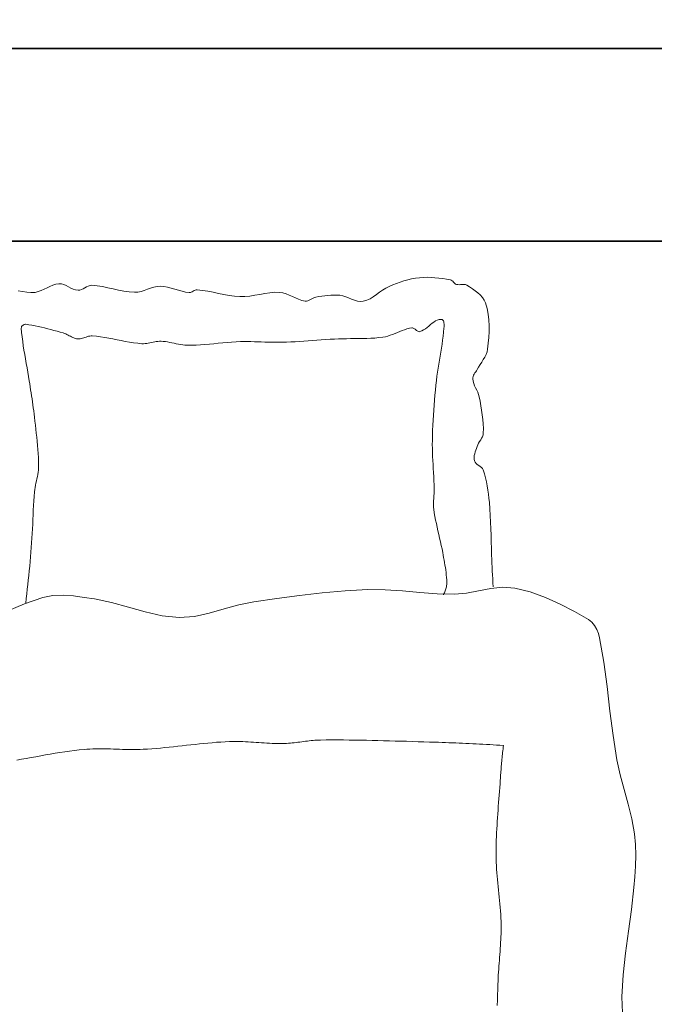
# Model space of a CAD drawing. Units: inches. Extents: x -36302355 to 648, y -221479757 to 75.
# Tile 35 of 37: x 311 to 341, y -20 to 26. Entities that reach past the tile are written whole.
import ezdxf

# ---------------------------------------------------------------- set-up
doc = ezdxf.new("R2010")
doc.units = ezdxf.units.IN
doc.header["$MEASUREMENT"] = 0
for name, color, linetype, lineweight in [('A-ANNO-DIMS', 2, 'Continuous', 18), ('A-FURN', 8, 'Continuous', 13), ('A-WALL', 7, 'Continuous', 35)]:
    doc.layers.add(name, color=color, linetype=linetype, lineweight=lineweight)
doc.styles.get("Standard").update_dxf_attribs({"font": 'arial.ttf'})
doc.dimstyles.get("Standard").update_dxf_attribs({"dimtxt": 0.18, "dimasz": 0.18, "dimexe": 0.18, "dimexo": 0.0625, "dimgap": 0.09, "dimtad": 0, "dimtih": 1, "dimtoh": 1, "dimdec": 0, "dimzin": 0, "dimdsep": 46, "dimlunit": 3, "dimtxsty": 'Standard', "dimcen": 0.09, "dimadec": 0, "dimazin": 0, "dimtfac": 1, "dimtdec": 0, "dimtofl": 0, "dimtmove": 0, "dimatfit": 3, "dimfxl": 1, "dimtolj": 1, "dimtzin": 0, "dimarcsym": 0})

# ---------------------------------------------------------------- blocks, each defined once
blk = doc.blocks.new('*D4')
at = {"layer": 'A-ANNO-DIMS', "color": 0, "lineweight": -2, "transparency": 16777216}
for p, q in [((145.197, 25.043), (145.197, 71.11)), ((145.377, 70.93), (364.803, 70.93)), ((605.017, 70.93), (385.59, 70.93)), ((605.197, 25.043), (605.197, 71.11))]:
    blk.add_line(p, q, dxfattribs=at)
at = {"layer": 'A-ANNO-DIMS', "color": 0, "transparency": 16777216}
for points in [[(145.377, 70.96), (145.377, 70.9), (145.197, 70.93)], [(605.017, 70.96), (605.017, 70.9), (605.197, 70.93)]]:
    blk.add_solid(points, dxfattribs=at)
at = {"layer": 'Defpoints', "color": 0, "transparency": 16777216}
for p in [(605.197, 70.93), (145.197, 24.981), (605.197, 24.981)]:
    blk.add_point(p, dxfattribs=at)
at = {"layer": 'A-ANNO-DIMS', "color": 0, "transparency": 16777216, "insert": (375.197, 70.93), "char_height": 6, "attachment_point": 5}
blk.add_mtext('\\A1;38\'-4"', dxfattribs=at)
blk = doc.blocks.new('BED-DOUBLE')
for p, q in [((29.019, 79.595), (28.885, 79.529)), ((29.156, 79.653), (29.019, 79.595)), ((29.295, 79.695), (29.156, 79.653)), ((29.439, 79.716), (29.295, 79.695)), ((29.555, 79.707), (29.439, 79.716)), ((29.667, 79.676), (29.555, 79.707)), ((29.776, 79.63), (29.667, 79.676)), ((29.885, 79.575), (29.776, 79.63)), ((30.811, 79.61), (30.732, 79.571)), ((30.892, 79.636), (30.811, 79.61)), ((30.976, 79.644), (30.892, 79.636)), ((31.228, 79.624), (30.976, 79.644)), ((31.477, 79.585), (31.228, 79.624)), ((34.02, 79.587), (33.869, 79.555)), ((34.173, 79.598), (34.02, 79.587)), ((34.345, 79.587), (34.173, 79.598)), ((34.515, 79.557), (34.345, 79.587)), ((44.859, 79.595), (44.703, 79.516)), ((45.03, 79.665), (44.859, 79.595)), ((45.203, 79.731), (45.03, 79.665)), ((45.378, 79.793), (45.203, 79.731)), ((45.554, 79.85), (45.378, 79.793)), ((45.733, 79.9), (45.554, 79.85)), ((45.912, 79.943), (45.733, 79.9)), ((46.094, 79.977), (45.912, 79.943)), ((46.276, 80.001), (46.094, 79.977)), ((46.457, 80.015), (46.276, 80.001)), ((46.638, 80.019), (46.457, 80.015)), ((46.819, 80.013), (46.638, 80.019)), ((47.001, 80.001), (46.819, 80.013)), ((47.182, 79.981), (47.001, 80.001)), ((47.363, 79.957), (47.182, 79.981)), ((47.542, 79.928), (47.363, 79.957)), ((47.721, 79.897), (47.542, 79.928)), ((47.762, 79.883), (47.721, 79.897)), ((47.799, 79.86), (47.762, 79.883)), ((47.832, 79.831), (47.799, 79.86)), ((47.865, 79.797), (47.832, 79.831)), ((47.897, 79.763), (47.865, 79.797)), ((47.93, 79.732), (47.897, 79.763)), ((47.966, 79.705), (47.93, 79.732)), ((48.005, 79.687), (47.966, 79.705)), ((48.065, 79.675), (48.005, 79.687)), ((48.126, 79.673), (48.065, 79.675)), ((48.189, 79.677), (48.126, 79.673)), ((48.253, 79.684), (48.189, 79.677)), ((48.316, 79.688), (48.253, 79.684)), ((48.376, 79.687), (48.316, 79.688)), ((48.434, 79.676), (48.376, 79.687)), ((48.487, 79.652), (48.434, 79.676)), ((48.617, 79.57), (48.487, 79.652)), ((27.733, 79.348), (27.532, 79.381)), ((27.935, 79.319), (27.733, 79.348)), ((28.135, 79.305), (27.935, 79.319)), ((28.332, 79.316), (28.135, 79.305)), ((28.475, 79.348), (28.332, 79.316)), ((28.614, 79.399), (28.475, 79.348)), ((28.75, 79.461), (28.614, 79.399)), ((28.885, 79.529), (28.75, 79.461)), ((29.994, 79.518), (29.885, 79.575)), ((30.103, 79.467), (29.994, 79.518)), ((30.215, 79.429), (30.103, 79.467)), ((30.331, 79.412), (30.215, 79.429)), ((30.415, 79.419), (30.331, 79.412)), ((30.496, 79.445), (30.415, 79.419)), ((30.575, 79.483), (30.496, 79.445)), ((30.654, 79.527), (30.575, 79.483)), ((30.732, 79.571), (30.654, 79.527)), ((31.725, 79.534), (31.477, 79.585)), ((31.973, 79.478), (31.725, 79.534)), ((32.221, 79.421), (31.973, 79.478)), ((32.469, 79.372), (32.221, 79.421)), ((32.718, 79.336), (32.469, 79.372)), ((32.97, 79.321), (32.718, 79.336)), ((33.123, 79.331), (32.97, 79.321)), ((33.273, 79.362), (33.123, 79.331)), ((33.423, 79.406), (33.273, 79.362)), ((33.571, 79.458), (33.423, 79.406)), ((33.72, 79.51), (33.571, 79.458)), ((33.869, 79.555), (33.72, 79.51)), ((34.684, 79.516), (34.515, 79.557)), ((34.852, 79.467), (34.684, 79.516)), ((35.02, 79.416), (34.852, 79.467)), ((35.188, 79.369), (35.02, 79.416)), ((35.358, 79.33), (35.188, 79.369)), ((35.529, 79.305), (35.358, 79.33)), ((35.577, 79.308), (35.529, 79.305)), ((35.623, 79.323), (35.577, 79.308)), ((35.669, 79.345), (35.623, 79.323)), ((35.714, 79.371), (35.669, 79.345)), ((35.758, 79.398), (35.714, 79.371)), ((35.804, 79.42), (35.758, 79.398)), ((35.85, 79.435), (35.804, 79.42)), ((35.898, 79.439), (35.85, 79.435)), ((36.149, 79.41), (35.898, 79.439)), ((36.398, 79.368), (36.149, 79.41)), ((36.646, 79.318), (36.398, 79.368)), ((36.894, 79.264), (36.646, 79.318)), ((37.142, 79.212), (36.894, 79.264)), ((37.39, 79.167), (37.142, 79.212)), ((37.64, 79.133), (37.39, 79.167)), ((37.891, 79.115), (37.64, 79.133)), ((38.357, 79.144), (38.124, 79.119)), ((38.588, 79.18), (38.357, 79.144)), ((38.82, 79.223), (38.588, 79.18)), ((39.051, 79.265), (38.82, 79.223)), ((39.283, 79.299), (39.051, 79.265)), ((39.515, 79.318), (39.283, 79.299)), ((39.748, 79.315), (39.515, 79.318)), ((39.902, 79.292), (39.748, 79.315)), ((40.051, 79.248), (39.902, 79.292)), ((40.198, 79.189), (40.051, 79.248)), ((40.343, 79.122), (40.198, 79.189)), ((41.721, 79.137), (41.582, 79.116)), ((41.86, 79.157), (41.721, 79.137)), ((42, 79.173), (41.86, 79.157)), ((42.139, 79.184), (42, 79.173)), ((42.279, 79.19), (42.139, 79.184)), ((42.419, 79.19), (42.279, 79.19)), ((42.558, 79.182), (42.419, 79.19)), ((42.698, 79.158), (42.558, 79.182)), ((42.835, 79.114), (42.698, 79.158)), ((44.266, 79.21), (44.121, 79.107)), ((44.409, 79.317), (44.266, 79.21)), ((44.554, 79.421), (44.409, 79.317)), ((44.703, 79.516), (44.554, 79.421)), ((48.749, 79.484), (48.617, 79.57)), ((48.879, 79.394), (48.749, 79.484)), ((49.004, 79.298), (48.879, 79.394)), ((49.119, 79.194), (49.004, 79.298)), ((49.219, 79.081), (49.119, 79.194)), ((38.124, 79.119), (37.891, 79.115)), ((40.488, 79.055), (40.343, 79.122)), ((40.634, 78.992), (40.488, 79.055)), ((40.783, 78.942), (40.634, 78.992)), ((40.936, 78.91), (40.783, 78.942)), ((41.002, 78.91), (40.936, 78.91)), ((41.066, 78.924), (41.002, 78.91)), ((41.128, 78.95), (41.066, 78.924)), ((41.19, 78.981), (41.128, 78.95)), ((41.252, 79.016), (41.19, 78.981)), ((41.315, 79.048), (41.252, 79.016)), ((41.378, 79.075), (41.315, 79.048)), ((41.444, 79.093), (41.378, 79.075)), ((41.582, 79.116), (41.444, 79.093)), ((42.971, 79.06), (42.835, 79.114)), ((43.106, 79.003), (42.971, 79.06)), ((43.241, 78.95), (43.106, 79.003)), ((43.377, 78.91), (43.241, 78.95)), ((43.513, 78.89), (43.377, 78.91)), ((43.651, 78.898), (43.513, 78.89)), ((43.817, 78.944), (43.651, 78.898)), ((43.972, 79.016), (43.817, 78.944)), ((44.121, 79.107), (43.972, 79.016)), ((49.301, 78.957), (49.219, 79.081)), ((49.36, 78.82), (49.301, 78.957)), ((49.432, 78.561), (49.36, 78.82)), ((49.482, 78.296), (49.432, 78.561)), ((49.513, 78.027), (49.482, 78.296)), ((27.712, 77.735), (27.728, 77.755)), ((27.728, 77.755), (27.746, 77.773)), ((27.746, 77.773), (27.767, 77.789)), ((27.767, 77.789), (27.789, 77.803)), ((27.789, 77.803), (27.812, 77.813)), ((27.812, 77.813), (27.835, 77.821)), ((27.835, 77.821), (27.858, 77.824)), ((27.858, 77.824), (27.88, 77.824)), ((27.88, 77.824), (28.029, 77.804)), ((28.029, 77.804), (28.178, 77.781)), ((28.178, 77.781), (28.326, 77.754)), ((28.326, 77.754), (28.474, 77.723)), ((46.713, 77.741), (46.79, 77.807)), ((46.79, 77.807), (46.868, 77.87)), ((46.868, 77.87), (46.947, 77.928)), ((46.947, 77.928), (47.028, 77.978)), ((47.028, 77.978), (47.112, 78.016)), ((47.112, 78.016), (47.2, 78.041)), ((47.2, 78.041), (47.293, 78.049)), ((47.293, 78.049), (47.337, 78.04)), ((47.337, 78.04), (47.371, 78.018)), ((47.371, 78.018), (47.396, 77.983)), ((47.396, 77.983), (47.413, 77.939)), ((47.413, 77.939), (47.423, 77.887)), ((47.423, 77.887), (47.427, 77.828)), ((47.427, 77.766), (47.424, 77.701)), ((47.427, 77.828), (47.427, 77.766)), ((49.527, 77.755), (49.513, 78.027)), ((49.526, 77.481), (49.527, 77.755)), ((27.683, 77.649), (27.684, 77.671)), ((27.699, 77.441), (27.683, 77.649)), ((27.684, 77.671), (27.689, 77.693)), ((27.689, 77.693), (27.699, 77.715)), ((27.699, 77.715), (27.712, 77.735)), ((27.721, 77.234), (27.699, 77.441)), ((28.474, 77.723), (28.621, 77.691)), ((28.621, 77.691), (28.768, 77.655)), ((28.768, 77.655), (28.915, 77.618)), ((28.915, 77.618), (29.061, 77.58)), ((29.061, 77.58), (29.206, 77.54)), ((29.206, 77.54), (29.352, 77.499)), ((29.352, 77.499), (29.497, 77.458)), ((29.497, 77.458), (29.643, 77.417)), ((29.643, 77.417), (29.7, 77.398)), ((29.7, 77.398), (29.757, 77.376)), ((29.757, 77.376), (29.813, 77.349)), ((29.813, 77.349), (29.867, 77.321)), ((29.867, 77.321), (29.922, 77.292)), ((29.922, 77.292), (29.977, 77.263)), ((44.799, 77.273), (44.912, 77.309)), ((44.912, 77.309), (45.023, 77.35)), ((45.023, 77.35), (45.135, 77.394)), ((45.135, 77.394), (45.245, 77.439)), ((45.245, 77.439), (45.356, 77.485)), ((45.356, 77.485), (45.467, 77.529)), ((45.467, 77.529), (45.579, 77.57)), ((45.579, 77.57), (45.692, 77.607)), ((45.692, 77.607), (45.806, 77.636)), ((45.806, 77.636), (45.922, 77.659)), ((45.922, 77.659), (45.956, 77.659)), ((45.956, 77.659), (45.988, 77.65)), ((45.988, 77.65), (46.02, 77.634)), ((46.02, 77.634), (46.051, 77.613)), ((46.051, 77.613), (46.082, 77.589)), ((46.082, 77.589), (46.112, 77.564)), ((46.112, 77.564), (46.142, 77.538)), ((46.142, 77.538), (46.172, 77.515)), ((46.172, 77.515), (46.203, 77.496)), ((46.203, 77.496), (46.234, 77.483)), ((46.234, 77.483), (46.266, 77.478)), ((46.266, 77.478), (46.299, 77.482)), ((46.299, 77.482), (46.388, 77.515)), ((46.388, 77.515), (46.473, 77.56)), ((46.473, 77.56), (46.555, 77.615)), ((46.555, 77.615), (46.635, 77.677)), ((46.635, 77.677), (46.713, 77.741)), ((47.4, 77.462), (47.383, 77.273)), ((47.405, 77.515), (47.4, 77.462)), ((47.412, 77.574), (47.405, 77.515)), ((47.418, 77.637), (47.412, 77.574)), ((47.424, 77.701), (47.418, 77.637)), ((49.513, 77.208), (49.526, 77.481)), ((27.746, 77.027), (27.721, 77.234)), ((27.776, 76.821), (27.746, 77.027)), ((29.977, 77.263), (30.031, 77.234)), ((30.031, 77.234), (30.086, 77.207)), ((30.086, 77.207), (30.142, 77.184)), ((30.142, 77.184), (30.199, 77.164)), ((30.199, 77.164), (30.257, 77.148)), ((30.257, 77.148), (30.316, 77.139)), ((30.316, 77.139), (30.374, 77.137)), ((30.374, 77.137), (30.43, 77.142)), ((30.43, 77.142), (30.487, 77.153)), ((30.487, 77.153), (30.543, 77.169)), ((30.543, 77.169), (30.599, 77.187)), ((30.599, 77.187), (30.656, 77.207)), ((30.656, 77.207), (30.712, 77.227)), ((30.712, 77.227), (30.768, 77.246)), ((30.768, 77.246), (30.824, 77.261)), ((30.824, 77.261), (30.881, 77.273)), ((30.881, 77.273), (30.938, 77.28)), ((30.938, 77.28), (30.995, 77.28)), ((30.995, 77.28), (31.19, 77.261)), ((31.19, 77.261), (31.384, 77.237)), ((31.384, 77.237), (31.577, 77.207)), ((31.577, 77.207), (31.77, 77.173)), ((31.77, 77.173), (31.963, 77.137)), ((31.963, 77.137), (32.155, 77.099)), ((32.155, 77.099), (32.348, 77.062)), ((32.348, 77.062), (32.54, 77.025)), ((32.54, 77.025), (32.733, 76.991)), ((32.733, 76.991), (32.927, 76.961)), ((32.927, 76.961), (33.12, 76.936)), ((33.12, 76.936), (33.315, 76.917)), ((33.315, 76.917), (33.39, 76.915)), ((33.39, 76.915), (33.465, 76.919)), ((33.465, 76.919), (33.54, 76.927)), ((33.54, 76.927), (33.614, 76.939)), ((33.614, 76.939), (33.689, 76.954)), ((33.689, 76.954), (33.763, 76.97)), ((33.763, 76.97), (33.838, 76.986)), ((33.838, 76.986), (33.912, 77.002)), ((33.912, 77.002), (33.987, 77.015)), ((33.987, 77.015), (34.062, 77.026)), ((34.062, 77.026), (34.137, 77.032)), ((34.137, 77.032), (34.212, 77.032)), ((34.212, 77.032), (34.314, 77.026)), ((34.314, 77.026), (34.416, 77.014)), ((34.416, 77.014), (34.517, 76.997)), ((34.517, 76.997), (34.618, 76.978)), ((34.618, 76.978), (34.718, 76.956)), ((34.718, 76.956), (34.819, 76.934)), ((34.819, 76.934), (34.92, 76.912)), ((34.92, 76.912), (35.02, 76.891)), ((35.02, 76.891), (35.121, 76.873)), ((35.121, 76.873), (35.223, 76.858)), ((35.223, 76.858), (35.324, 76.848)), ((35.324, 76.848), (35.426, 76.845)), ((35.426, 76.845), (35.634, 76.847)), ((35.634, 76.847), (35.842, 76.854)), ((35.842, 76.854), (36.05, 76.866)), ((36.05, 76.866), (36.258, 76.881)), ((36.258, 76.881), (36.465, 76.899)), ((36.465, 76.899), (36.673, 76.918)), ((36.673, 76.918), (36.88, 76.938)), ((36.88, 76.938), (37.088, 76.957)), ((37.088, 76.957), (37.296, 76.976)), ((37.296, 76.976), (37.503, 76.992)), ((37.503, 76.992), (37.711, 77.005)), ((37.711, 77.005), (37.919, 77.014)), ((37.919, 77.014), (38.081, 77.017)), ((38.081, 77.017), (38.242, 77.017)), ((38.242, 77.017), (38.404, 77.015)), ((38.404, 77.015), (38.566, 77.011)), ((38.566, 77.011), (38.727, 77.006)), ((38.727, 77.006), (38.889, 77)), ((38.889, 77), (39.051, 76.993)), ((39.051, 76.993), (39.212, 76.988)), ((39.212, 76.988), (39.374, 76.984)), ((39.374, 76.984), (39.536, 76.981)), ((39.536, 76.981), (39.697, 76.981)), ((39.697, 76.981), (39.859, 76.984)), ((39.859, 76.984), (40.063, 76.991)), ((40.063, 76.991), (40.267, 77)), ((40.267, 77), (40.471, 77.011)), ((40.471, 77.011), (40.675, 77.024)), ((40.675, 77.024), (40.879, 77.038)), ((40.879, 77.038), (41.082, 77.053)), ((41.082, 77.053), (41.286, 77.068)), ((41.286, 77.068), (41.49, 77.083)), ((41.49, 77.083), (41.694, 77.098)), ((41.694, 77.098), (41.898, 77.112)), ((41.898, 77.112), (42.102, 77.125)), ((42.102, 77.125), (42.306, 77.136)), ((42.306, 77.136), (42.494, 77.144)), ((42.494, 77.144), (42.683, 77.148)), ((42.683, 77.148), (42.872, 77.151)), ((42.872, 77.151), (43.061, 77.152)), ((43.061, 77.152), (43.25, 77.152)), ((43.25, 77.152), (43.439, 77.153)), ((43.439, 77.153), (43.628, 77.156)), ((43.628, 77.156), (43.817, 77.161)), ((43.817, 77.161), (44.005, 77.169)), ((44.005, 77.169), (44.193, 77.181)), ((44.193, 77.181), (44.381, 77.199)), ((44.381, 77.199), (44.568, 77.222)), ((44.568, 77.222), (44.684, 77.244)), ((44.684, 77.244), (44.799, 77.273)), ((47.334, 76.896), (47.305, 76.708)), ((47.36, 77.084), (47.334, 76.896)), ((47.383, 77.273), (47.36, 77.084)), ((49.459, 76.667), (49.49, 76.936)), ((49.49, 76.936), (49.513, 77.208)), ((27.808, 76.615), (27.776, 76.821)), ((27.843, 76.41), (27.808, 76.615)), ((27.879, 76.204), (27.843, 76.41)), ((47.273, 76.52), (47.241, 76.333)), ((47.305, 76.708), (47.273, 76.52)), ((49.327, 76.292), (49.387, 76.412)), ((49.387, 76.412), (49.432, 76.537)), ((49.432, 76.537), (49.459, 76.667)), ((27.915, 75.999), (27.879, 76.204)), ((27.952, 75.793), (27.915, 75.999)), ((47.175, 75.958), (47.144, 75.77)), ((47.208, 76.145), (47.175, 75.958)), ((47.241, 76.333), (47.208, 76.145)), ((49.036, 75.827), (49.108, 75.944)), ((49.108, 75.944), (49.184, 76.059)), ((49.184, 76.059), (49.258, 76.175)), ((49.258, 76.175), (49.327, 76.292)), ((27.987, 75.588), (27.952, 75.793)), ((28.021, 75.382), (27.987, 75.588)), ((47.115, 75.582), (47.089, 75.394)), ((47.144, 75.77), (47.115, 75.582)), ((48.806, 75.441), (48.836, 75.495)), ((48.836, 75.495), (48.871, 75.549)), ((48.871, 75.549), (48.907, 75.602)), ((48.907, 75.602), (48.941, 75.655)), ((48.941, 75.655), (48.971, 75.709)), ((48.971, 75.709), (49.036, 75.827)), ((28.053, 75.176), (28.021, 75.382)), ((28.074, 75.036), (28.053, 75.176)), ((28.095, 74.896), (28.074, 75.036)), ((47.068, 75.205), (47.044, 74.972)), ((47.089, 75.394), (47.068, 75.205)), ((48.764, 75.269), (48.767, 75.329)), ((48.781, 75.161), (48.764, 75.269)), ((48.767, 75.329), (48.782, 75.386)), ((48.812, 75.056), (48.781, 75.161)), ((48.782, 75.386), (48.806, 75.441)), ((48.854, 74.954), (48.812, 75.056)), ((28.117, 74.755), (28.095, 74.896)), ((28.139, 74.615), (28.117, 74.755)), ((28.161, 74.475), (28.139, 74.615)), ((47.022, 74.739), (47.001, 74.505)), ((47.044, 74.972), (47.022, 74.739)), ((48.901, 74.853), (48.854, 74.954)), ((48.95, 74.751), (48.901, 74.853)), ((48.996, 74.649), (48.95, 74.751)), ((49.036, 74.546), (48.996, 74.649)), ((49.064, 74.439), (49.036, 74.546)), ((28.182, 74.335), (28.161, 74.475)), ((28.203, 74.194), (28.182, 74.335)), ((28.224, 74.054), (28.203, 74.194)), ((46.981, 74.272), (46.962, 74.038)), ((47.001, 74.505), (46.981, 74.272)), ((49.105, 74.229), (49.064, 74.439)), ((49.144, 74.017), (49.105, 74.229)), ((28.243, 73.914), (28.224, 74.054)), ((28.262, 73.773), (28.243, 73.914)), ((28.279, 73.632), (28.262, 73.773)), ((28.296, 73.491), (28.279, 73.632)), ((46.945, 73.805), (46.929, 73.571)), ((46.962, 74.038), (46.945, 73.805)), ((49.181, 73.805), (49.144, 74.017)), ((49.212, 73.592), (49.181, 73.805)), ((28.317, 73.302), (28.296, 73.491)), ((28.339, 73.113), (28.317, 73.302)), ((46.916, 73.337), (46.904, 73.103)), ((46.929, 73.571), (46.916, 73.337)), ((49.238, 73.379), (49.212, 73.592)), ((49.255, 73.166), (49.238, 73.379)), ((49.263, 72.952), (49.255, 73.166)), ((28.361, 72.924), (28.339, 73.113)), ((28.383, 72.734), (28.361, 72.924)), ((28.404, 72.545), (28.383, 72.734)), ((46.894, 72.869), (46.886, 72.635)), ((46.904, 73.103), (46.894, 72.869)), ((49.248, 72.654), (49.26, 72.738)), ((49.26, 72.738), (49.263, 72.952)), ((28.424, 72.356), (28.404, 72.545)), ((28.442, 72.166), (28.424, 72.356)), ((46.88, 72.401), (46.878, 72.212)), ((46.886, 72.635), (46.88, 72.401)), ((48.998, 72.191), (49.04, 72.269)), ((49.04, 72.269), (49.087, 72.345)), ((49.087, 72.345), (49.136, 72.42)), ((49.136, 72.42), (49.181, 72.496)), ((49.181, 72.496), (49.22, 72.573)), ((49.22, 72.573), (49.248, 72.654)), ((28.458, 71.976), (28.442, 72.166)), ((28.471, 71.786), (28.458, 71.976)), ((28.482, 71.596), (28.471, 71.786)), ((46.878, 72.212), (46.88, 72.024)), ((46.88, 72.024), (46.885, 71.835)), ((46.885, 71.835), (46.892, 71.647)), ((48.837, 71.692), (48.856, 71.777)), ((48.856, 71.777), (48.88, 71.861)), ((48.88, 71.861), (48.909, 71.945)), ((48.909, 71.945), (48.938, 72.028)), ((48.938, 72.028), (48.965, 72.11)), ((48.965, 72.11), (48.998, 72.191)), ((28.488, 71.406), (28.482, 71.596)), ((28.491, 71.216), (28.488, 71.406)), ((46.892, 71.647), (46.902, 71.458)), ((46.902, 71.458), (46.912, 71.27)), ((48.827, 71.607), (48.837, 71.692)), ((48.828, 71.523), (48.827, 71.607)), ((48.842, 71.44), (48.828, 71.523)), ((48.872, 71.375), (48.842, 71.44)), ((48.919, 71.32), (48.872, 71.375)), ((48.978, 71.271), (48.919, 71.32)), ((28.451, 70.81), (28.467, 70.911)), ((28.467, 70.911), (28.48, 71.012)), ((28.48, 71.012), (28.488, 71.114)), ((28.488, 71.114), (28.491, 71.216)), ((46.912, 71.27), (46.923, 71.081)), ((46.923, 71.081), (46.934, 70.893)), ((46.934, 70.893), (46.944, 70.704)), ((49.043, 71.226), (48.978, 71.271)), ((49.109, 71.182), (49.043, 71.226)), ((49.17, 71.134), (49.109, 71.182)), ((49.221, 71.08), (49.17, 71.134)), ((49.256, 71.016), (49.221, 71.08)), ((49.316, 70.833), (49.256, 71.016)), ((28.348, 70.306), (28.368, 70.407)), ((28.368, 70.407), (28.389, 70.508)), ((28.389, 70.508), (28.411, 70.608)), ((28.411, 70.608), (28.432, 70.709)), ((28.432, 70.709), (28.451, 70.81)), ((46.944, 70.704), (46.954, 70.516)), ((46.954, 70.516), (46.961, 70.327)), ((49.367, 70.648), (49.316, 70.833)), ((49.409, 70.46), (49.367, 70.648)), ((49.445, 70.27), (49.409, 70.46)), ((28.285, 69.785), (28.303, 70.002)), ((28.303, 70.002), (28.315, 70.104)), ((28.315, 70.104), (28.33, 70.205)), ((28.33, 70.205), (28.348, 70.306)), ((46.964, 69.98), (46.959, 69.901)), ((46.961, 70.327), (46.966, 70.138)), ((46.966, 70.059), (46.964, 69.98)), ((46.966, 70.138), (46.966, 70.059)), ((49.474, 70.079), (49.445, 70.27)), ((49.499, 69.887), (49.474, 70.079)), ((28.256, 69.35), (28.27, 69.568)), ((28.27, 69.568), (28.285, 69.785)), ((46.932, 69.506), (46.93, 69.427)), ((46.936, 69.585), (46.932, 69.506)), ((46.941, 69.664), (46.936, 69.585)), ((46.947, 69.743), (46.941, 69.664)), ((46.954, 69.822), (46.947, 69.743)), ((46.959, 69.901), (46.954, 69.822)), ((49.521, 69.695), (49.499, 69.887)), ((49.541, 69.503), (49.521, 69.695)), ((49.567, 69.196), (49.541, 69.503)), ((28.234, 68.915), (28.244, 69.133)), ((28.244, 69.133), (28.256, 69.35)), ((46.93, 69.427), (46.93, 69.349)), ((46.93, 69.349), (46.934, 69.27)), ((46.934, 69.27), (46.943, 69.192)), ((46.943, 69.192), (46.968, 69.02)), ((46.968, 69.02), (46.997, 68.85)), ((49.586, 68.889), (49.567, 69.196)), ((28.213, 68.48), (28.223, 68.697)), ((28.223, 68.697), (28.234, 68.915)), ((46.997, 68.85), (47.03, 68.679)), ((47.03, 68.679), (47.066, 68.51)), ((49.6, 68.581), (49.586, 68.889)), ((49.611, 68.273), (49.6, 68.581)), ((28.192, 68.045), (28.203, 68.262)), ((28.203, 68.262), (28.213, 68.48)), ((47.066, 68.51), (47.103, 68.34)), ((47.103, 68.34), (47.142, 68.171)), ((47.142, 68.171), (47.182, 68.002)), ((49.619, 67.964), (49.611, 68.273)), ((28.166, 67.61), (28.18, 67.827)), ((28.18, 67.827), (28.192, 68.045)), ((47.182, 68.002), (47.221, 67.833)), ((47.221, 67.833), (47.26, 67.664)), ((47.26, 67.664), (47.297, 67.495)), ((49.627, 67.656), (49.619, 67.964)), ((49.636, 67.348), (49.627, 67.656)), ((28.113, 66.959), (28.132, 67.176)), ((28.132, 67.176), (28.15, 67.392)), ((28.15, 67.392), (28.166, 67.61)), ((47.297, 67.495), (47.332, 67.325)), ((47.332, 67.325), (47.364, 67.155)), ((49.647, 67.04), (49.636, 67.348)), ((28.074, 66.526), (28.094, 66.742)), ((28.094, 66.742), (28.113, 66.959)), ((47.364, 67.155), (47.385, 67.039)), ((47.385, 67.039), (47.406, 66.924)), ((47.406, 66.924), (47.428, 66.809)), ((47.428, 66.809), (47.448, 66.693)), ((49.655, 66.854), (49.647, 67.04)), ((49.664, 66.668), (49.655, 66.854)), ((28.032, 66.093), (28.053, 66.309)), ((28.053, 66.309), (28.074, 66.526)), ((47.448, 66.693), (47.468, 66.577)), ((47.468, 66.577), (47.487, 66.462)), ((47.487, 66.462), (47.504, 66.346)), ((47.504, 66.346), (47.519, 66.23)), ((49.672, 66.482), (49.664, 66.668)), ((49.68, 66.296), (49.672, 66.482)), ((49.689, 66.11), (49.68, 66.296)), ((27.987, 65.66), (28.01, 65.876)), ((28.01, 65.876), (28.032, 66.093)), ((47.519, 66.23), (47.532, 66.113)), ((47.532, 66.113), (47.543, 65.997)), ((47.543, 65.997), (47.55, 65.88)), ((47.55, 65.88), (47.554, 65.763)), ((49.697, 65.924), (49.689, 66.11)), ((49.706, 65.738), (49.697, 65.924)), ((27.938, 65.228), (27.963, 65.444)), ((27.963, 65.444), (27.987, 65.66)), ((42.802, 65.366), (41.735, 65.273)), ((43.87, 65.425), (42.802, 65.366)), ((44.678, 65.422), (43.87, 65.425)), ((45.485, 65.369), (44.678, 65.422)), ((46.292, 65.296), (45.485, 65.369)), ((47.484, 65.367), (47.466, 65.32)), ((47.501, 65.415), (47.484, 65.367)), ((47.515, 65.464), (47.501, 65.415)), ((47.527, 65.513), (47.515, 65.464)), ((47.537, 65.563), (47.527, 65.513)), ((47.545, 65.613), (47.537, 65.563)), ((47.55, 65.663), (47.545, 65.613)), ((47.553, 65.713), (47.55, 65.663)), ((47.554, 65.763), (47.553, 65.713)), ((49.04, 65.369), (48.474, 65.264)), ((49.604, 65.477), (49.04, 65.369)), ((50.166, 65.538), (49.604, 65.477)), ((49.715, 65.552), (49.706, 65.738)), ((50.724, 65.499), (50.166, 65.538)), ((51.45, 65.318), (50.724, 65.499)), ((28.68, 65.056), (27.839, 64.768)), ((27.887, 64.796), (27.913, 65.012)), ((27.913, 65.012), (27.938, 65.228)), ((29.152, 65.148), (28.68, 65.056)), ((29.636, 65.165), (29.152, 65.148)), ((30.126, 65.13), (29.636, 65.165)), ((30.616, 65.064), (30.126, 65.13)), ((31.101, 64.99), (30.616, 65.064)), ((31.896, 64.828), (31.101, 64.99)), ((39.609, 65.014), (38.549, 64.862)), ((40.671, 65.153), (39.609, 65.014)), ((41.735, 65.273), (40.671, 65.153)), ((47.1, 65.235), (46.292, 65.296)), ((47.908, 65.214), (47.1, 65.235)), ((47.422, 65.229), (47.397, 65.186)), ((47.445, 65.274), (47.422, 65.229)), ((47.466, 65.32), (47.445, 65.274)), ((48.474, 65.264), (47.908, 65.214)), ((52.158, 65.065), (51.45, 65.318)), ((52.846, 64.755), (52.158, 65.065)), ((27.839, 64.768), (27.022, 64.416)), ((32.683, 64.608), (31.896, 64.828)), ((33.469, 64.384), (32.683, 64.608)), ((37.155, 64.522), (36.463, 64.326)), ((37.849, 64.716), (37.155, 64.522)), ((38.549, 64.862), (37.849, 64.716)), ((53.517, 64.405), (52.846, 64.755)), ((54.172, 64.032), (53.517, 64.405)), ((34.259, 64.206), (33.469, 64.384)), ((35.061, 64.125), (34.259, 64.206)), ((35.767, 64.177), (35.061, 64.125)), ((36.463, 64.326), (35.767, 64.177)), ((54.33, 63.91), (54.172, 64.032)), ((54.459, 63.752), (54.33, 63.91)), ((54.561, 63.57), (54.459, 63.752)), ((54.638, 63.375), (54.561, 63.57)), ((54.689, 63.176), (54.638, 63.375)), ((54.886, 62.042), (54.689, 63.176)), ((55.039, 60.9), (54.886, 62.042)), ((55.175, 59.755), (55.039, 60.9)), ((55.318, 58.611), (55.175, 59.755)), ((55.495, 57.473), (55.318, 58.611)), ((30.75, 57.972), (30.613, 57.96)), ((30.888, 57.98), (30.75, 57.972)), ((31.026, 57.986), (30.888, 57.98)), ((31.163, 57.989), (31.026, 57.986)), ((31.301, 57.991), (31.163, 57.989)), ((31.439, 57.99), (31.301, 57.991)), ((31.577, 57.988), (31.439, 57.99)), ((31.716, 57.985), (31.577, 57.988)), ((31.854, 57.981), (31.716, 57.985)), ((31.992, 57.977), (31.854, 57.981)), ((32.13, 57.972), (31.992, 57.977)), ((32.268, 57.967), (32.13, 57.972)), ((32.407, 57.963), (32.268, 57.967)), ((33.373, 57.965), (33.235, 57.959)), ((33.576, 57.978), (33.373, 57.965)), ((33.778, 57.992), (33.576, 57.978)), ((33.98, 58.008), (33.778, 57.992)), ((34.182, 58.026), (33.98, 58.008)), ((34.384, 58.045), (34.182, 58.026)), ((34.586, 58.065), (34.384, 58.045)), ((34.788, 58.087), (34.586, 58.065)), ((34.989, 58.108), (34.788, 58.087)), ((35.191, 58.131), (34.989, 58.108)), ((35.393, 58.153), (35.191, 58.131)), ((35.594, 58.175), (35.393, 58.153)), ((35.796, 58.197), (35.594, 58.175)), ((35.998, 58.218), (35.796, 58.197)), ((36.2, 58.239), (35.998, 58.218)), ((36.401, 58.258), (36.2, 58.239)), ((36.603, 58.276), (36.401, 58.258)), ((36.806, 58.292), (36.603, 58.276)), ((37.008, 58.306), (36.806, 58.292)), ((37.21, 58.318), (37.008, 58.306)), ((37.413, 58.327), (37.21, 58.318)), ((37.537, 58.331), (37.413, 58.327)), ((37.661, 58.333), (37.537, 58.331)), ((37.785, 58.332), (37.661, 58.333)), ((37.909, 58.329), (37.785, 58.332)), ((38.034, 58.325), (37.909, 58.329)), ((38.158, 58.319), (38.034, 58.325)), ((38.282, 58.313), (38.158, 58.319)), ((38.406, 58.305), (38.282, 58.313)), ((38.53, 58.296), (38.406, 58.305)), ((38.654, 58.288), (38.53, 58.296)), ((38.779, 58.279), (38.654, 58.288)), ((38.903, 58.27), (38.779, 58.279)), ((39.027, 58.261), (38.903, 58.27)), ((39.151, 58.253), (39.027, 58.261)), ((39.275, 58.246), (39.151, 58.253)), ((39.4, 58.241), (39.275, 58.246)), ((39.524, 58.236), (39.4, 58.241)), ((39.648, 58.233), (39.524, 58.236)), ((39.772, 58.232), (39.648, 58.233)), ((39.896, 58.233), (39.772, 58.232)), ((39.985, 58.235), (39.896, 58.233)), ((40.073, 58.24), (39.985, 58.235)), ((40.162, 58.246), (40.073, 58.24)), ((40.25, 58.254), (40.162, 58.246)), ((40.338, 58.262), (40.25, 58.254)), ((40.426, 58.272), (40.338, 58.262)), ((40.514, 58.283), (40.426, 58.272)), ((40.603, 58.294), (40.514, 58.283)), ((40.691, 58.306), (40.603, 58.294)), ((40.779, 58.318), (40.691, 58.306)), ((40.867, 58.33), (40.779, 58.318)), ((40.955, 58.342), (40.867, 58.33)), ((41.043, 58.353), (40.955, 58.342)), ((41.131, 58.363), (41.043, 58.353)), ((41.219, 58.373), (41.131, 58.363)), ((41.307, 58.381), (41.219, 58.373)), ((41.395, 58.389), (41.307, 58.381)), ((41.484, 58.394), (41.395, 58.389)), ((41.572, 58.398), (41.484, 58.394)), ((41.661, 58.4), (41.572, 58.398)), ((41.928, 58.402), (41.661, 58.4)), ((42.196, 58.402), (41.928, 58.402)), ((42.464, 58.402), (42.196, 58.402)), ((42.731, 58.401), (42.464, 58.402)), ((42.999, 58.398), (42.731, 58.401)), ((43.267, 58.395), (42.999, 58.398)), ((43.535, 58.391), (43.267, 58.395)), ((43.802, 58.386), (43.535, 58.391)), ((44.07, 58.381), (43.802, 58.386)), ((44.338, 58.375), (44.07, 58.381)), ((44.605, 58.368), (44.338, 58.375)), ((44.873, 58.362), (44.605, 58.368)), ((45.141, 58.354), (44.873, 58.362)), ((45.408, 58.346), (45.141, 58.354)), ((45.676, 58.339), (45.408, 58.346)), ((45.944, 58.33), (45.676, 58.339)), ((46.211, 58.322), (45.944, 58.33)), ((46.479, 58.314), (46.211, 58.322)), ((46.746, 58.306), (46.479, 58.314)), ((47.014, 58.298), (46.746, 58.306)), ((47.173, 58.293), (47.014, 58.298)), ((47.333, 58.287), (47.173, 58.293)), ((47.492, 58.282), (47.333, 58.287)), ((47.651, 58.276), (47.492, 58.282)), ((47.81, 58.27), (47.651, 58.276)), ((47.97, 58.263), (47.81, 58.27)), ((48.129, 58.257), (47.97, 58.263)), ((48.288, 58.25), (48.129, 58.257)), ((48.447, 58.242), (48.288, 58.25)), ((48.606, 58.235), (48.447, 58.242)), ((48.766, 58.227), (48.606, 58.235)), ((48.925, 58.219), (48.766, 58.227)), ((49.084, 58.21), (48.925, 58.219)), ((49.243, 58.201), (49.084, 58.21)), ((49.402, 58.192), (49.243, 58.201)), ((49.561, 58.183), (49.402, 58.192)), ((49.72, 58.173), (49.561, 58.183)), ((49.879, 58.163), (49.72, 58.173)), ((50.038, 58.153), (49.879, 58.163)), ((50.197, 58.142), (50.038, 58.153)), ((50.17, 57.9), (50.179, 57.981)), ((50.179, 57.981), (50.188, 58.062)), ((50.188, 58.062), (50.197, 58.142)), ((27.916, 57.542), (27.691, 57.503)), ((28.14, 57.582), (27.916, 57.542)), ((28.364, 57.622), (28.14, 57.582)), ((28.588, 57.662), (28.364, 57.622)), ((28.812, 57.702), (28.588, 57.662)), ((29.036, 57.741), (28.812, 57.702)), ((29.261, 57.778), (29.036, 57.741)), ((29.485, 57.815), (29.261, 57.778)), ((29.71, 57.849), (29.485, 57.815)), ((29.935, 57.881), (29.71, 57.849)), ((30.161, 57.91), (29.935, 57.881)), ((30.386, 57.937), (30.161, 57.91)), ((30.613, 57.96), (30.386, 57.937)), ((32.545, 57.959), (32.407, 57.963)), ((32.683, 57.956), (32.545, 57.959)), ((32.821, 57.954), (32.683, 57.956)), ((32.959, 57.954), (32.821, 57.954)), ((33.097, 57.956), (32.959, 57.954)), ((33.235, 57.959), (33.097, 57.956)), ((50.129, 57.497), (50.137, 57.577)), ((50.137, 57.577), (50.145, 57.658)), ((50.145, 57.658), (50.153, 57.739)), ((50.153, 57.739), (50.162, 57.82)), ((50.162, 57.82), (50.17, 57.9)), ((27.691, 57.503), (27.467, 57.465)), ((50.086, 57.012), (50.093, 57.092)), ((50.093, 57.092), (50.1, 57.173)), ((50.1, 57.173), (50.107, 57.254)), ((50.107, 57.254), (50.114, 57.335)), ((50.114, 57.335), (50.122, 57.416)), ((50.122, 57.416), (50.129, 57.497)), ((55.646, 56.779), (55.495, 57.473)), ((50.051, 56.526), (50.056, 56.607)), ((50.056, 56.607), (50.062, 56.688)), ((50.062, 56.688), (50.068, 56.769)), ((50.068, 56.769), (50.074, 56.85)), ((50.074, 56.85), (50.08, 56.931)), ((50.08, 56.931), (50.086, 57.012)), ((55.831, 56.091), (55.646, 56.779)), ((50.013, 56), (50.026, 56.175)), ((50.026, 56.175), (50.039, 56.35)), ((50.039, 56.35), (50.051, 56.526)), ((49.987, 55.649), (50, 55.824)), ((50, 55.824), (50.013, 56)), ((56.024, 55.406), (55.831, 56.091)), ((49.947, 55.123), (49.96, 55.298)), ((49.96, 55.298), (49.973, 55.474)), ((49.973, 55.474), (49.987, 55.649)), ((56.197, 54.717), (56.024, 55.406)), ((49.91, 54.596), (49.922, 54.772)), ((49.922, 54.772), (49.934, 54.947)), ((49.934, 54.947), (49.947, 55.123)), ((49.89, 54.245), (49.9, 54.421)), ((49.9, 54.421), (49.91, 54.596)), ((56.323, 54.019), (56.197, 54.717)), ((49.867, 53.719), (49.873, 53.894)), ((49.873, 53.894), (49.881, 54.07)), ((49.881, 54.07), (49.89, 54.245)), ((56.369, 53.519), (56.323, 54.019)), ((49.857, 53.192), (49.859, 53.367)), ((49.859, 53.367), (49.862, 53.543)), ((49.862, 53.543), (49.867, 53.719)), ((56.379, 53.016), (56.369, 53.519)), ((49.857, 53.016), (49.857, 53.192)), ((49.859, 52.853), (49.857, 53.016)), ((56.363, 52.512), (56.379, 53.016)), ((49.865, 52.69), (49.859, 52.853)), ((49.872, 52.527), (49.865, 52.69)), ((49.882, 52.365), (49.872, 52.527)), ((56.33, 52.008), (56.363, 52.512)), ((49.894, 52.202), (49.882, 52.365)), ((49.907, 52.04), (49.894, 52.202)), ((49.922, 51.877), (49.907, 52.04)), ((56.292, 51.505), (56.33, 52.008)), ((49.938, 51.715), (49.922, 51.877)), ((49.954, 51.553), (49.938, 51.715)), ((49.971, 51.39), (49.954, 51.553)), ((49.988, 51.228), (49.971, 51.39)), ((50.004, 51.065), (49.988, 51.228)), ((50.02, 50.903), (50.004, 51.065)), ((56.186, 50.484), (56.292, 51.505)), ((50.035, 50.741), (50.02, 50.903)), ((50.049, 50.578), (50.035, 50.741)), ((50.062, 50.416), (50.049, 50.578)), ((50.072, 50.253), (50.062, 50.416)), ((50.081, 50.09), (50.072, 50.253)), ((56.047, 49.466), (56.186, 50.484)), ((50.087, 49.927), (50.081, 50.09)), ((50.091, 49.764), (50.087, 49.927)), ((50.092, 49.626), (50.091, 49.764)), ((50.083, 49.211), (50.088, 49.349)), ((50.088, 49.349), (50.091, 49.488)), ((50.091, 49.488), (50.092, 49.626)), ((55.905, 48.448), (56.047, 49.466)), ((50.051, 48.658), (50.061, 48.797)), ((50.061, 48.797), (50.069, 48.935)), ((50.069, 48.935), (50.077, 49.073)), ((50.077, 49.073), (50.083, 49.211)), ((50.02, 48.244), (50.031, 48.382)), ((50.031, 48.382), (50.041, 48.52)), ((50.041, 48.52), (50.051, 48.658)), ((55.79, 47.428), (55.905, 48.448)), ((49.987, 47.83), (49.998, 47.968)), ((49.998, 47.968), (50.009, 48.106)), ((50.009, 48.106), (50.02, 48.244)), ((49.952, 47.277), (49.959, 47.415)), ((49.959, 47.415), (49.968, 47.553)), ((49.968, 47.553), (49.977, 47.691)), ((49.977, 47.691), (49.987, 47.83)), ((55.733, 46.404), (55.79, 47.428)), ((49.934, 46.749), (49.941, 47)), ((49.941, 47), (49.946, 47.138)), ((49.946, 47.138), (49.952, 47.277)), ((49.92, 46.246), (49.927, 46.497)), ((49.927, 46.497), (49.934, 46.749)), ((49.913, 45.995), (49.92, 46.246)), ((55.763, 45.66), (55.733, 46.404))]:
    blk.add_line(p, q)

msp = doc.modelspace()

# ---------------------------------------------------------------- linework, layer by layer
at = {"layer": 'A-WALL'}
for p, q in [((145.197, 24.981), (605.197, 24.981)), ((145.197, 15.981), (605.197, 15.981))]:
    msp.add_line(p, q, dxfattribs=at)

# ---------------------------------------------------------------- block references
at = {"layer": 'A-FURN'}
msp.add_blockref('BED-DOUBLE', (283.833, -65.73), dxfattribs=at)

# ---------------------------------------------------------------- dimensions: what is measured, and where the dimension line sits
at = {"layer": 'A-ANNO-DIMS'}
dim = msp.add_linear_dim(base=(605.197, 70.93), p1=(145.197, 24.981), p2=(605.197, 24.981), dimstyle='Standard', override={"dimtxt": 6, "dimclrd": 0, "dimclre": 0, "dimclrt": 0}, dxfattribs=at)
dim.commit()
dim.dimension.update_dxf_attribs({"geometry": '*D4', "text_midpoint": (375.197, 70.93)})

doc.saveas('drawing.dxf')
